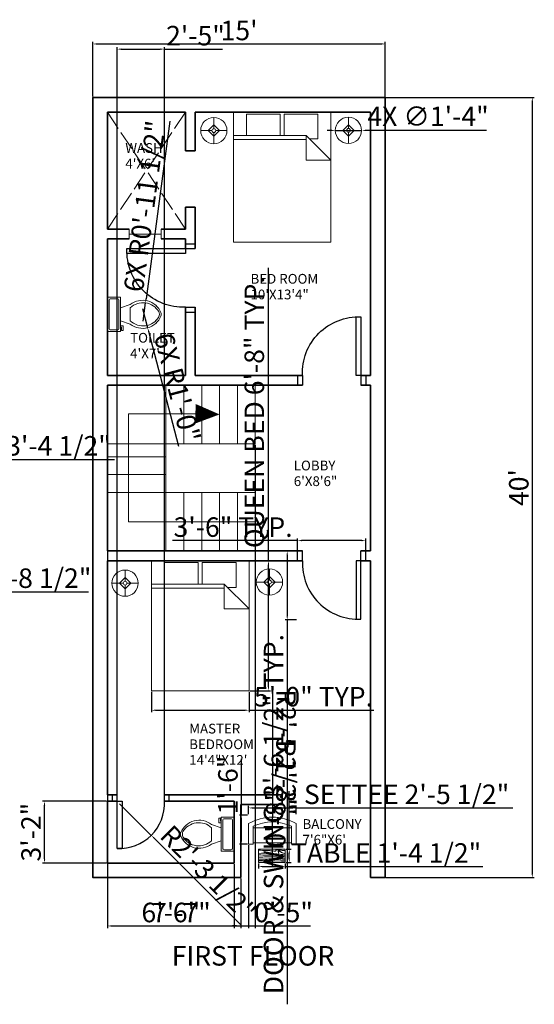
# Model space of a CAD drawing. Units: inches. Extents: x 2353 to 2961, y 642 to 1248.
# Tile 5 of 5: x 2644 to 2961, y 642 to 1248. Entities that reach past the tile are written whole.
import ezdxf

# ---------------------------------------------------------------- set-up
doc = ezdxf.new("R2010")
doc.units = ezdxf.units.IN
doc.linetypes.add('ACAD_ISO02W100', pattern=[15, 12, -3])
for name, color, linetype, lineweight in [('A-ANNO-DIMS', 2, 'Continuous', 18), ('A-ANNO-TEXT', 7, 'Continuous', 25), ('A-AREA-IDEN', 7, 'Continuous', 18), ('A-DOOR', 4, 'Continuous', 25), ('A-FLOR-FIXT', 9, 'Continuous', 18), ('A-FLOR-OPEN', 8, 'ACAD_ISO02W100', 13), ('A-FLOR-STRS', 7, 'Continuous', 18), ('A-FURN', 8, 'Continuous', 18), ('A-GLAZ', 4, 'Continuous', 18), ('A-WALL', 7, 'Continuous', 35)]:
    doc.layers.add(name, color=color, linetype=linetype, lineweight=lineweight)
doc.styles.get("Standard").update_dxf_attribs({"font": 'arial.ttf'})
doc.dimstyles.new('ISO-25', dxfattribs={"dimtxt": 12, "dimasz": 2.5, "dimexe": 1.25, "dimexo": 0.625, "dimtad": 1, "dimdec": 1, "dimlunit": 3, "dimtxsty": 'Standard', "dimcen": 2.5, "dimadec": 0, "dimazin": 0, "dimtfac": 1, "dimtdec": 1, "dimtmove": 0, "dimatfit": 3, "dimfxl": 1, "dimarcsym": 0})

# ---------------------------------------------------------------- blocks, each defined once
blk = doc.blocks.new('*D9')
at = {"layer": 'A-ANNO-DIMS', "color": 0, "lineweight": -2, "transparency": 16777216}
for p, q in [((2870.09, 1199.98), (2961.19, 1199.98)), ((2959.94, 1197.48), (2959.94, 722.48)), ((2870.09, 719.98), (2961.19, 719.98))]:
    blk.add_line(p, q, dxfattribs=at)
at = {"layer": 'A-ANNO-DIMS', "color": 0, "transparency": 16777216}
for points in [[(2959.53, 1197.48), (2960.36, 1197.48), (2959.94, 1199.98)], [(2959.53, 722.48), (2960.36, 722.48), (2959.94, 719.98)]]:
    blk.add_solid(points, dxfattribs=at)
at = {"layer": 'Defpoints', "color": 0, "transparency": 16777216}
for p in [(2869.46, 1199.98), (2869.46, 719.98), (2959.94, 719.98)]:
    blk.add_point(p, dxfattribs=at)
at = {"layer": 'A-ANNO-DIMS', "color": 0, "transparency": 16777216, "insert": (2953.19, 959.98), "char_height": 12, "attachment_point": 5, "rotation": 90}
blk.add_mtext("40'", dxfattribs=at)
blk = doc.blocks.new('Sofa - Roundback Loveseat 5 ft.')
for p, q in [((-24, -33.99998), (-24, -11.46958)), ((0, -32.44198), (0, -5.99998)), ((24.00004, -33.99998), (24.00004, -11.46958)), ((-23.9998, -13.38178), (23.99986, -13.38178)), ((-24, -32.44198), (24.00004, -32.44198))]:
    blk.add_line(p, q)
for points in [[(-24, -33.99998), (-30, -33.99998), (-30, -7.99998)], [(30.00004, -7.99998), (30.00004, -33.99998), (24.00004, -33.99998)]]:
    blk.add_lwpolyline(points)
for centre, radius, start, end in [((0, -60.24998), 60.24998, 60.13715, 119.8628), ((0, -61.38438), 55.38444, 64.32083, 115.6792)]:
    blk.add_arc(centre, radius, start, end)
blk = doc.blocks.new('Bed - Queen')
for p, q in [((0, -80.00003), (0, 0)), ((0, 0), (59.99999, 0)), ((59.99999, 0), (59.99999, -80.00003)), ((7.99999, -1.2), (28.79998, -1.2)), ((7.99999, -14.4), (7.99999, -1.2)), ((28.79998, -1.2), (28.79998, -14.4)), ((31.19999, -1.2), (51.99999, -1.2)), ((31.19999, -14.4), (31.19999, -1.2)), ((51.99999, -1.2), (51.99999, -16.4)), ((0, -14.4), (44.8, -14.4)), ((44.8, -16.8), (0, -16.8)), ((59.99999, -29.6), (44.8, -14.4)), ((44.8, -14.4), (44.8, -29.6)), ((51.99999, -16.4), (46.79936, -16.4)), ((44.8, -29.6), (59.99999, -29.6)), ((59.99999, -80.00003), (0, -80.00003))]:
    blk.add_line(p, q)
blk = doc.blocks.new('Lamp - Table')
for p, q in [((0, 7), (0, 1)), ((-1, 0), (-7, 0)), ((0, 3), (-3, 0)), ((-3, 0), (0, -3)), ((3, 0), (0, 3)), ((0, -3), (3, 0)), ((1, 0), (7, 0)), ((0, -1), (0, -7))]:
    blk.add_line(p, q)
for radius in [7, 1]:
    blk.add_circle((0, 0), radius)
blk = doc.blocks.new('Toilet - top')
for p, q in [((9.5, -6), (9.5, -2)), ((-10, -8.5), (-8, -8.5)), ((-10, -9.5), (-10, -8.5)), ((-7, -9.5), (-10, -9.5)), ((-8, -8.5), (-8, -8)), ((-7, -8), (-7, -9.5)), ((-4, -8), (-6, -14)), ((4, -8), (6, -14)), ((4, -14), (-4, -14))]:
    blk.add_line(p, q)
blk.add_lwpolyline([(10.5, -8), (10.5, 0), (-10.5, 0), (-10.5, -8)], close=True)
for points in [[(-9.5, -2), (-9.5, -6)], [(8.5, -1), (-8.5, -1)], [(-8.5, -7), (8.5, -7)]]:
    blk.add_lwpolyline(points)
for centre, radius, start, end in [((-8.62, -1.88), 0.884, 81.8699, 188.1301), ((-8.62, -6.12), 0.884, 171.8699, 278.1301), ((8.62, -1.88), 0.884, 351.8699, 98.1301), ((8.62, -6.12), 0.884, 261.8699, 8.1301), ((3.52, -21.58), 12.17, 141.46911, 247.97143), ((4.2, -21.82), 11.33, 136.36773, 238.94682), ((-3.52, -21.58), 12.17, 292.02843, 38.53071), ((-4.2, -21.82), 11.33, 301.05301, 43.63209), ((0, -27.88), 4, 245.73182, 294.26817), ((0, -29), 4, 254.86053, 285.13947)]:
    blk.add_arc(centre, radius, start, end)
blk = doc.blocks.new('Table - Rectangular Woodgrain 60 x 30 in.')
for p, q in [((0, 0), (0, -30)), ((60, 0), (0, 0)), ((60, -30), (60, 0)), ((0, -30), (60, -30))]:
    blk.add_line(p, q)
for points in [[(0, -2.4), (4.8155, -2.418), (9.0302, -2.4688), (12.709, -2.5477), (15.9167, -2.65), (18.7181, -2.7711), (21.1781, -2.9063), (23.3616, -3.0508), (25.3333, -3.2), (27.1477, -3.3495), (28.8172, -3.4958), (30.3437, -3.636), (31.7291, -3.7667), (32.9756, -3.8849), (34.0849, -3.9875), (35.059, -4.0714), (35.9, -4.1334), (36.6114, -4.1711), (37.2041, -4.1854), (37.6906, -4.1779), (38.0833, -4.15), (38.3948, -4.1034), (38.6375, -4.0396), (38.8239, -3.9602), (38.9666, -3.8667), (39.0764, -3.7608), (39.1573, -3.6448), (39.2116, -3.521), (39.2416, -3.3917), (39.2498, -3.2593), (39.2385, -3.1261), (39.21, -2.9944), (39.1666, -2.8667), (39.111, -2.7447), (39.0468, -2.6281), (38.978, -2.5163), (38.9083, -2.4083), (38.8418, -2.3035), (38.7823, -2.201), (38.7337, -2.1001), (38.7, -2), (38.6844, -1.9003), (38.6875, -1.8021), (38.7094, -1.707), (38.75, -1.6167), (38.8094, -1.5326), (38.8875, -1.4563), (38.9844, -1.3893), (39.1, -1.3333), (39.2351, -1.2896), (39.3937, -1.2583), (39.5804, -1.2396), (39.8, -1.2333), (40.057, -1.2396), (40.3562, -1.2583), (40.7023, -1.2896), (41.1, -1.3333), (41.5547, -1.3895), (42.0755, -1.4573), (42.6721, -1.5361), (43.3542, -1.625), (44.1316, -1.7233), (45.014, -1.8302), (46.0114, -1.9449), (47.1333, -2.0667), (48.3862, -2.1947), (49.7625, -2.3281), (51.2513, -2.4663), (52.8416, -2.6083), (54.5226, -2.7535), (56.2833, -2.9011), (58.1127, -3.0501), (60, -3.2)], [(0, -9.2), (6.5759, -9.0858), (11.9385, -9.0365), (16.2527, -9.0418), (19.6833, -9.0917), (22.3952, -9.1759), (24.5531, -9.2844), (26.322, -9.4069), (27.8666, -9.5333), (29.3241, -9.6553), (30.7203, -9.7719), (32.0532, -9.8837), (33.3208, -9.9917), (34.5213, -10.0965), (35.6526, -10.199), (36.7128, -10.2999), (37.7, -10.4), (38.6129, -10.4996), (39.4531, -10.5969), (40.223, -10.6895), (40.925, -10.775), (41.5613, -10.8512), (42.1344, -10.9156), (42.6465, -10.966), (43.1, -11), (43.4976, -11.0158), (43.8437, -11.0136), (44.143, -10.9942), (44.4, -10.9583), (44.6195, -10.9069), (44.8062, -10.8406), (44.9648, -10.7603), (45.1, -10.6667), (45.2155, -10.5598), (45.3114, -10.4365), (45.3871, -10.2929), (45.4416, -10.125), (45.4743, -9.929), (45.4844, -9.7011), (45.4709, -9.4371), (45.4333, -9.1333), (45.3716, -8.7883), (45.2896, -8.4104), (45.1919, -8.0107), (45.0833, -7.6), (44.9685, -7.1893), (44.8521, -6.7896), (44.7388, -6.4117), (44.6333, -6.0667), (44.54, -5.7628), (44.4614, -5.4979), (44.4001, -5.2675), (44.3583, -5.0667), (44.3384, -4.8909), (44.3427, -4.7354), (44.3736, -4.5956), (44.4333, -4.4667), (44.5236, -4.3453), (44.6427, -4.2333), (44.7884, -4.1339), (44.9583, -4.05), (45.1501, -3.9849), (45.3614, -3.9417), (45.59, -3.9234), (45.8333, -3.9333), (46.0915, -3.9749), (46.3734, -4.0531), (46.6906, -4.1736), (47.0542, -4.3417), (47.4756, -4.5629), (47.9661, -4.8427), (48.5372, -5.1866), (49.2, -5.6), (49.9676, -6.0844), (50.8594, -6.625), (51.8965, -7.2031), (53.1, -7.8), (54.491, -8.3969), (56.0906, -8.975), (57.9199, -9.5156), (60, -10)], [(0, -12.8), (5.1847, -12.9322), (9.6213, -13.0323), (13.3963, -13.1059), (16.5958, -13.1583), (19.3063, -13.1952), (21.614, -13.2219), (23.6054, -13.2439), (25.3666, -13.2667), (26.9728, -13.2947), (28.4531, -13.3281), (29.8256, -13.3663), (31.1083, -13.4083), (32.3191, -13.4535), (33.476, -13.501), (34.597, -13.5501), (35.7, -13.6), (36.7984, -13.6497), (37.8875, -13.6979), (38.9578, -13.743), (40, -13.7833), (41.0047, -13.8174), (41.9625, -13.8438), (42.864, -13.8607), (43.7, -13.8667), (44.4631, -13.8604), (45.1552, -13.8417), (45.7801, -13.8104), (46.3416, -13.7667), (46.8439, -13.7104), (47.2906, -13.6417), (47.6858, -13.5604), (48.0333, -13.4667), (48.3375, -13.3608), (48.6042, -13.2448), (48.8396, -13.121), (49.05, -12.9917), (49.2417, -12.8593), (49.4208, -12.7261), (49.5937, -12.5944), (49.7667, -12.4667), (49.9452, -12.3451), (50.1323, -12.2313), (50.3303, -12.1268), (50.5416, -12.0333), (50.7686, -11.9524), (51.0135, -11.8854), (51.2788, -11.8341), (51.5666, -11.8), (51.8785, -11.7843), (52.2116, -11.7865), (52.562, -11.8059), (52.926, -11.8417), (53.2998, -11.8931), (53.6795, -11.9594), (54.0614, -12.0397), (54.4416, -12.1333), (54.8223, -12.2401), (55.2293, -12.3625), (55.6942, -12.5037), (56.2489, -12.6667), (56.9251, -12.8547), (57.7545, -13.0708), (58.7689, -13.3182), (60, -13.6)], [(0, -18), (5.124, -17.7273), (9.6609, -17.5057), (13.6705, -17.3303), (17.2125, -17.1958), (20.3467, -17.0973), (23.1328, -17.0297), (25.6307, -16.9878), (27.9, -16.9667), (29.9928, -16.9617), (31.9302, -16.9703), (33.7254, -16.9907), (35.3917, -17.0208), (36.9423, -17.0588), (38.3906, -17.1026), (39.7499, -17.1503), (41.0333, -17.2), (42.2519, -17.2496), (43.4073, -17.2969), (44.4986, -17.3395), (45.525, -17.375), (46.4858, -17.4012), (47.3802, -17.4156), (48.2074, -17.416), (48.9667, -17.4), (49.6583, -17.3662), (50.2872, -17.3167), (50.8595, -17.2547), (51.3812, -17.1833), (51.8584, -17.1057), (52.2971, -17.025), (52.7034, -16.9443), (53.0833, -16.8667), (53.443, -16.7951), (53.789, -16.7313), (54.128, -16.6768), (54.4666, -16.6334), (54.8115, -16.6024), (55.1693, -16.5854), (55.5465, -16.5841), (55.95, -16.6), (56.3828, -16.6337), (56.8346, -16.6823), (57.2915, -16.7418), (57.7396, -16.8084), (58.165, -16.878), (58.5539, -16.9469), (58.8924, -17.0111), (59.1666, -17.0667), (59.3679, -17.1107), (59.5078, -17.1438), (59.6032, -17.1675), (59.6708, -17.1833), (59.7275, -17.193), (59.7901, -17.1979), (59.8753, -17.1998), (60, -17.2)], [(0, -22.4), (8.0098, -22.2501), (14.4094, -22.1011), (19.4168, -21.9535), (23.25, -21.8083), (26.1269, -21.6663), (28.2656, -21.5281), (29.884, -21.3947), (31.2, -21.2667), (32.3967, -21.1448), (33.5172, -21.0292), (34.5697, -20.9198), (35.5625, -20.8167), (36.5037, -20.7198), (37.4015, -20.6292), (38.2642, -20.5448), (39.1, -20.4667), (39.9164, -20.3951), (40.7187, -20.3313), (41.5117, -20.2768), (42.3, -20.2333), (43.0883, -20.2024), (43.8812, -20.1854), (44.6836, -20.1841), (45.5, -20.2), (46.3328, -20.234), (47.1747, -20.2844), (48.0163, -20.3488), (48.8479, -20.425), (49.66, -20.5106), (50.4429, -20.6031), (51.1872, -20.7004), (51.8833, -20.8), (52.5246, -20.8999), (53.1166, -20.9995), (53.6681, -21.0983), (54.1875, -21.1958), (54.6834, -21.2919), (55.1646, -21.3859), (55.6394, -21.4777), (56.1167, -21.5667), (56.6028, -21.6515), (57.0961, -21.7266), (57.5929, -21.7852), (58.0896, -21.8208), (58.5823, -21.8268), (59.0674, -21.7964), (59.5412, -21.723), (60, -21.6)], [(0, -25.2), (8.6355, -25.0504), (15.7026, -24.9031), (21.4049, -24.7606), (25.9458, -24.625), (29.529, -24.4988), (32.3578, -24.3844), (34.6359, -24.284), (36.5667, -24.2), (38.3213, -24.1341), (39.9417, -24.0854), (41.437, -24.0523), (42.8167, -24.0333), (44.0901, -24.0268), (45.2667, -24.0313), (46.3557, -24.0451), (47.3667, -24.0667), (48.309, -24.0947), (49.1928, -24.1287), (50.0284, -24.168), (50.826, -24.2125), (51.5959, -24.2617), (52.3483, -24.3151), (53.0935, -24.3725), (53.8417, -24.4334), (54.6009, -24.497), (55.3699, -24.561), (56.1454, -24.6226), (56.9239, -24.6792), (57.7021, -24.7279), (58.4764, -24.7662), (59.2435, -24.7911), (60, -24.8)], [(0, -28.8), (5.6867, -28.6681), (10.45, -28.5698), (14.407, -28.5012), (17.675, -28.4584), (20.3711, -28.4374), (22.6125, -28.4344), (24.5164, -28.4455), (26.2, -28.4667), (27.762, -28.4947), (29.2276, -28.5281), (30.6033, -28.5663), (31.8958, -28.6084), (33.1118, -28.6535), (34.2578, -28.7011), (35.3405, -28.7501), (36.3666, -28.8), (37.3443, -28.8497), (38.288, -28.8974), (39.2137, -28.9412), (40.1375, -28.9792), (41.0753, -29.0093), (42.0432, -29.0297), (43.0572, -29.0384), (44.1333, -29.0333), (45.2936, -29.0114), (46.5843, -28.9641), (48.0579, -28.8816), (49.7666, -28.7542), (51.7629, -28.5721), (54.0989, -28.3255), (56.8272, -28.0048), (60, -27.6)]]:
    blk.add_lwpolyline(points)
blk = doc.blocks.new('*D11')
at = {"layer": 'A-ANNO-DIMS', "color": 0, "lineweight": -2, "transparency": 16777216}
for p, q in [((2689.46, 1200.61), (2689.46, 1234.16)), ((2691.96, 1232.91), (2866.96, 1232.91)), ((2869.46, 1200.61), (2869.46, 1234.16))]:
    blk.add_line(p, q, dxfattribs=at)
at = {"layer": 'A-ANNO-DIMS', "color": 0, "transparency": 16777216}
for points in [[(2691.96, 1233.33), (2691.96, 1232.49), (2689.46, 1232.91)], [(2866.96, 1233.33), (2866.96, 1232.49), (2869.46, 1232.91)]]:
    blk.add_solid(points, dxfattribs=at)
at = {"layer": 'Defpoints', "color": 0, "transparency": 16777216}
for p in [(2869.46, 1232.91), (2689.46, 1199.98), (2869.46, 1199.98)]:
    blk.add_point(p, dxfattribs=at)
at = {"layer": 'A-ANNO-DIMS', "color": 0, "transparency": 16777216, "insert": (2779.46, 1239.66), "char_height": 12, "attachment_point": 5}
blk.add_mtext("15'", dxfattribs=at)
blk = doc.blocks.new('DOOR-SINGLE-36IN')
for p, q in [((0, 6), (0, 0)), ((3, 6), (3, 0)), ((39, 6), (39, 0)), ((42, 6), (42, 0))]:
    blk.add_line(p, q)
blk.add_lwpolyline([(3, 6), (6, 6), (6, 42), (3, 42)], close=True)
blk.add_arc((4.5, 7.5), 34.53, 357.51045, 92.48955)
blk = doc.blocks.new('WASH-COURT-CROSS-4X6')
for p, q in [((0, 72), (48, 0)), ((48, 72), (0, 0))]:
    blk.add_line(p, q)
blk = doc.blocks.new('*D15')
at = {"layer": 'A-ANNO-DIMS', "color": 0, "lineweight": -2, "transparency": 16777216}
for p, q in [((2814.84, 920.98), (2807.85, 920.98)), ((2809.1, 918.48), (2809.1, 881.06)), ((2814.84, 878.56), (2807.85, 878.56)), ((2809.1, 878.56), (2809.1, 642.05))]:
    blk.add_line(p, q, dxfattribs=at)
at = {"layer": 'A-ANNO-DIMS', "color": 0, "transparency": 16777216}
for points in [[(2808.69, 918.48), (2809.52, 918.48), (2809.1, 920.98)], [(2808.69, 881.06), (2809.52, 881.06), (2809.1, 878.56)]]:
    blk.add_solid(points, dxfattribs=at)
at = {"layer": 'Defpoints', "color": 0, "transparency": 16777216}
for p in [(2815.46, 920.98), (2809.1, 878.56), (2815.46, 878.56)]:
    blk.add_point(p, dxfattribs=at)
at = {"layer": 'A-ANNO-DIMS', "color": 0, "transparency": 16777216, "insert": (2802.23, 759.06), "char_height": 12, "attachment_point": 5, "rotation": 90}
blk.add_mtext('DOOR & SWING 3\'-6 1/2" TYP.', dxfattribs=at)
blk = doc.blocks.new('*D16')
at = {"layer": 'A-ANNO-DIMS', "color": 0, "lineweight": -2, "transparency": 16777216}
for p, q in [((2815.46, 927.35), (2738.58, 927.35)), ((2815.46, 921.61), (2815.46, 928.6)), ((2854.96, 927.35), (2817.96, 927.35)), ((2857.46, 921.61), (2857.46, 928.6))]:
    blk.add_line(p, q, dxfattribs=at)
at = {"layer": 'A-ANNO-DIMS', "color": 0, "transparency": 16777216}
for points in [[(2817.96, 927.76), (2817.96, 926.93), (2815.46, 927.35)], [(2854.96, 927.76), (2854.96, 926.93), (2857.46, 927.35)]]:
    blk.add_solid(points, dxfattribs=at)
at = {"layer": 'Defpoints', "color": 0, "transparency": 16777216}
for p in [(2815.46, 927.35), (2815.46, 920.98), (2857.46, 920.98)]:
    blk.add_point(p, dxfattribs=at)
at = {"layer": 'A-ANNO-DIMS', "color": 0, "transparency": 16777216, "insert": (2775.77, 934.1), "char_height": 12, "attachment_point": 5}
blk.add_mtext('3\'-6" TYP.', dxfattribs=at)
blk = doc.blocks.new('*D17')
at = {"layer": 'A-ANNO-DIMS', "color": 0, "lineweight": -2, "transparency": 16777216}
for p, q in [((2797.58, 914.98), (2797.58, 1095.26)), ((2786.2, 914.98), (2798.83, 914.98)), ((2797.58, 837.48), (2797.58, 912.48)), ((2786.2, 834.98), (2798.83, 834.98))]:
    blk.add_line(p, q, dxfattribs=at)
at = {"layer": 'A-ANNO-DIMS', "color": 0, "transparency": 16777216}
for points in [[(2797.16, 912.48), (2797.99, 912.48), (2797.58, 914.98)], [(2797.16, 837.48), (2797.99, 837.48), (2797.58, 834.98)]]:
    blk.add_solid(points, dxfattribs=at)
at = {"layer": 'Defpoints', "color": 0, "transparency": 16777216}
for p in [(2785.58, 914.98), (2797.58, 914.98), (2785.58, 834.98)]:
    blk.add_point(p, dxfattribs=at)
at = {"layer": 'A-ANNO-DIMS', "color": 0, "transparency": 16777216, "insert": (2790.38, 1006.37), "char_height": 12, "attachment_point": 5, "rotation": 90}
blk.add_mtext('QUEEN BED 6\'-8" TYP.', dxfattribs=at)
blk = doc.blocks.new('*D18')
at = {"layer": 'A-ANNO-DIMS', "color": 0, "lineweight": -2, "transparency": 16777216}
for p, q in [((2725.58, 834.36), (2725.58, 821.73)), ((2785.58, 834.36), (2785.58, 821.73)), ((2728.08, 822.98), (2783.08, 822.98)), ((2785.58, 822.98), (2862.47, 822.98))]:
    blk.add_line(p, q, dxfattribs=at)
at = {"layer": 'A-ANNO-DIMS', "color": 0, "transparency": 16777216}
for points in [[(2728.08, 823.4), (2728.08, 822.57), (2725.58, 822.98)], [(2783.08, 823.4), (2783.08, 822.57), (2785.58, 822.98)]]:
    blk.add_solid(points, dxfattribs=at)
at = {"layer": 'Defpoints', "color": 0, "transparency": 16777216}
for p in [(2725.58, 834.98), (2785.58, 834.98), (2785.58, 822.98)]:
    blk.add_point(p, dxfattribs=at)
at = {"layer": 'A-ANNO-DIMS', "color": 0, "transparency": 16777216, "insert": (2825.27, 829.74), "char_height": 12, "attachment_point": 5}
blk.add_mtext('5\'-0" TYP.', dxfattribs=at)
blk = doc.blocks.new('*D21')
at = {"layer": 'A-ANNO-DIMS', "color": 0, "lineweight": -2, "transparency": 16777216}
for p, q in [((2529.01, 971.84), (2529.01, 978.53)), ((2531.51, 977.28), (2566.89, 977.28)), ((2569.39, 971.84), (2569.39, 978.53)), ((2569.39, 977.28), (2702.81, 977.28))]:
    blk.add_line(p, q, dxfattribs=at)
at = {"layer": 'A-ANNO-DIMS', "color": 0, "transparency": 16777216}
for points in [[(2531.51, 977.69), (2531.51, 976.86), (2529.01, 977.28)], [(2566.89, 977.69), (2566.89, 976.86), (2569.39, 977.28)]]:
    blk.add_solid(points, dxfattribs=at)
at = {"layer": 'Defpoints', "color": 0, "transparency": 16777216}
for p in [(2569.39, 977.28), (2529.01, 971.22), (2569.39, 971.22)]:
    blk.add_point(p, dxfattribs=at)
at = {"layer": 'A-ANNO-DIMS', "color": 0, "transparency": 16777216, "insert": (2637.35, 984.11), "char_height": 12, "attachment_point": 5}
blk.add_mtext('SETTEE 3\'-4 1/2"', dxfattribs=at)
blk = doc.blocks.new('*D23')
at = {"layer": 'A-ANNO-DIMS', "color": 0, "lineweight": -2, "transparency": 16777216}
for p, q in [((2785.29, 759.09), (2785.29, 764.12)), ((2814.63, 759.09), (2814.63, 764.12)), ((2787.79, 762.87), (2812.13, 762.87)), ((2814.63, 762.87), (2948.05, 762.87))]:
    blk.add_line(p, q, dxfattribs=at)
at = {"layer": 'A-ANNO-DIMS', "color": 0, "transparency": 16777216}
for points in [[(2787.79, 763.28), (2787.79, 762.45), (2785.29, 762.87)], [(2812.13, 763.28), (2812.13, 762.45), (2814.63, 762.87)]]:
    blk.add_solid(points, dxfattribs=at)
at = {"layer": 'Defpoints', "color": 0, "transparency": 16777216}
for p in [(2785.29, 758.46), (2814.63, 762.87), (2814.63, 758.46)]:
    blk.add_point(p, dxfattribs=at)
at = {"layer": 'A-ANNO-DIMS', "color": 0, "transparency": 16777216, "insert": (2882.59, 769.7), "char_height": 12, "attachment_point": 5}
blk.add_mtext('SETTEE 2\'-5 1/2"', dxfattribs=at)
blk = doc.blocks.new('*D24')
at = {"layer": 'A-ANNO-DIMS', "color": 0, "lineweight": -2, "transparency": 16777216}
for p, q in [((2780.89, 758.46), (2780.89, 792.98)), ((2784.67, 758.46), (2779.64, 758.46)), ((2780.89, 743.03), (2780.89, 755.96)), ((2784.67, 740.53), (2779.64, 740.53))]:
    blk.add_line(p, q, dxfattribs=at)
at = {"layer": 'A-ANNO-DIMS', "color": 0, "transparency": 16777216}
for points in [[(2780.47, 755.96), (2781.31, 755.96), (2780.89, 758.46)], [(2780.47, 743.03), (2781.31, 743.03), (2780.89, 740.53)]]:
    blk.add_solid(points, dxfattribs=at)
at = {"layer": 'Defpoints', "color": 0, "transparency": 16777216}
for p in [(2780.89, 758.46), (2785.29, 758.46), (2785.29, 740.53)]:
    blk.add_point(p, dxfattribs=at)
at = {"layer": 'A-ANNO-DIMS', "color": 0, "transparency": 16777216, "insert": (2774.14, 776.97), "char_height": 12, "attachment_point": 5, "rotation": 90}
blk.add_mtext('1\'-6"', dxfattribs=at)
blk = doc.blocks.new('*D27')
at = {"layer": 'A-ANNO-DIMS', "color": 0, "lineweight": -2, "transparency": 16777216}
for p, q in [((2791.43, 728.61), (2791.43, 725.52)), ((2807.88, 728.61), (2807.88, 725.52)), ((2793.93, 726.77), (2805.38, 726.77)), ((2807.88, 726.77), (2929.56, 726.77))]:
    blk.add_line(p, q, dxfattribs=at)
at = {"layer": 'A-ANNO-DIMS', "color": 0, "transparency": 16777216}
for points in [[(2793.93, 727.19), (2793.93, 726.35), (2791.43, 726.77)], [(2805.38, 727.19), (2805.38, 726.35), (2807.88, 726.77)]]:
    blk.add_solid(points, dxfattribs=at)
at = {"layer": 'Defpoints', "color": 0, "transparency": 16777216}
for p in [(2791.43, 729.24), (2807.88, 729.24), (2807.88, 726.77)]:
    blk.add_point(p, dxfattribs=at)
at = {"layer": 'A-ANNO-DIMS', "color": 0, "transparency": 16777216, "insert": (2869.97, 733.6), "char_height": 12, "attachment_point": 5}
blk.add_mtext('TABLE 1\'-4 1/2"', dxfattribs=at)
blk = doc.blocks.new('*D28')
at = {"layer": 'A-ANNO-DIMS', "color": 0, "lineweight": -2, "transparency": 16777216}
for p, q in [((2810.35, 737.46), (2810.35, 773.11)), ((2808.5, 737.46), (2811.6, 737.46)), ((2810.35, 731.74), (2810.35, 734.96)), ((2808.5, 729.24), (2811.6, 729.24))]:
    blk.add_line(p, q, dxfattribs=at)
at = {"layer": 'A-ANNO-DIMS', "color": 0, "transparency": 16777216}
for points in [[(2809.93, 734.96), (2810.76, 734.96), (2810.35, 737.46)], [(2809.93, 731.74), (2810.76, 731.74), (2810.35, 729.24)]]:
    blk.add_solid(points, dxfattribs=at)
at = {"layer": 'Defpoints', "color": 0, "transparency": 16777216}
for p in [(2807.88, 737.46), (2810.35, 737.46), (2807.88, 729.24)]:
    blk.add_point(p, dxfattribs=at)
at = {"layer": 'A-ANNO-DIMS', "color": 0, "transparency": 16777216, "insert": (2803.6, 756.54), "char_height": 12, "attachment_point": 5, "rotation": 90}
blk.add_mtext('0\'-8"', dxfattribs=at)
blk = doc.blocks.new('*D33')
at = {"layer": 'A-ANNO-DIMS', "color": 0, "lineweight": -2, "transparency": 16777216}
for p, q in [((2698.46, 728.36), (2698.46, 688.98)), ((2776.46, 728.36), (2776.46, 688.98)), ((2700.96, 690.23), (2773.96, 690.23))]:
    blk.add_line(p, q, dxfattribs=at)
at = {"layer": 'A-ANNO-DIMS', "color": 0, "transparency": 16777216}
for points in [[(2700.96, 690.65), (2700.96, 689.82), (2698.46, 690.23)], [(2773.96, 690.65), (2773.96, 689.82), (2776.46, 690.23)]]:
    blk.add_solid(points, dxfattribs=at)
at = {"layer": 'Defpoints', "color": 0, "transparency": 16777216}
for p in [(2698.46, 728.98), (2776.46, 728.98), (2776.46, 690.23)]:
    blk.add_point(p, dxfattribs=at)
at = {"layer": 'A-ANNO-DIMS', "color": 0, "transparency": 16777216, "insert": (2737.46, 696.99), "char_height": 12, "attachment_point": 5}
blk.add_mtext('6\'-6"', dxfattribs=at)
blk = doc.blocks.new('*D34')
at = {"layer": 'A-ANNO-DIMS', "color": 0, "lineweight": -2, "transparency": 16777216}
for p, q in [((2697.84, 766.98), (2658.46, 766.98)), ((2659.71, 731.48), (2659.71, 764.48)), ((2697.84, 728.98), (2658.46, 728.98))]:
    blk.add_line(p, q, dxfattribs=at)
at = {"layer": 'A-ANNO-DIMS', "color": 0, "transparency": 16777216}
for points in [[(2659.3, 764.48), (2660.13, 764.48), (2659.71, 766.98)], [(2659.3, 731.48), (2660.13, 731.48), (2659.71, 728.98)]]:
    blk.add_solid(points, dxfattribs=at)
at = {"layer": 'Defpoints', "color": 0, "transparency": 16777216}
for p in [(2659.71, 766.98), (2698.46, 766.98), (2698.46, 728.98)]:
    blk.add_point(p, dxfattribs=at)
at = {"layer": 'A-ANNO-DIMS', "color": 0, "transparency": 16777216, "insert": (2652.96, 747.98), "char_height": 12, "attachment_point": 5, "rotation": 90}
blk.add_mtext('3\'-2"', dxfattribs=at)
blk = doc.blocks.new('*D37')
at = {"layer": 'A-ANNO-DIMS', "color": 0, "lineweight": -2, "transparency": 16777216}
for p, q in [((2698.46, 986.36), (2698.46, 688.98)), ((2789.46, 986.36), (2789.46, 688.98)), ((2700.96, 690.23), (2786.96, 690.23))]:
    blk.add_line(p, q, dxfattribs=at)
at = {"layer": 'A-ANNO-DIMS', "color": 0, "transparency": 16777216}
for points in [[(2700.96, 690.65), (2700.96, 689.82), (2698.46, 690.23)], [(2786.96, 690.65), (2786.96, 689.82), (2789.46, 690.23)]]:
    blk.add_solid(points, dxfattribs=at)
at = {"layer": 'Defpoints', "color": 0, "transparency": 16777216}
for p in [(2698.46, 986.98), (2789.46, 986.98), (2789.46, 690.23)]:
    blk.add_point(p, dxfattribs=at)
at = {"layer": 'A-ANNO-DIMS', "color": 0, "transparency": 16777216, "insert": (2743.96, 696.86), "char_height": 12, "attachment_point": 5}
blk.add_mtext('7\'-7"', dxfattribs=at)
blk = doc.blocks.new('*D39')
at = {"layer": 'A-ANNO-DIMS', "color": 0, "lineweight": -2, "transparency": 16777216}
for p, q in [((2704.46, 767.61), (2704.46, 1230.98)), ((2733.46, 767.61), (2733.46, 1230.98)), ((2706.96, 1229.73), (2730.96, 1229.73)), ((2733.46, 1229.73), (2769.32, 1229.73))]:
    blk.add_line(p, q, dxfattribs=at)
at = {"layer": 'A-ANNO-DIMS', "color": 0, "transparency": 16777216}
for points in [[(2706.96, 1230.15), (2706.96, 1229.32), (2704.46, 1229.73)], [(2730.96, 1230.15), (2730.96, 1229.32), (2733.46, 1229.73)]]:
    blk.add_solid(points, dxfattribs=at)
at = {"layer": 'Defpoints', "color": 0, "transparency": 16777216}
for p in [(2733.46, 1229.73), (2704.46, 766.98), (2733.46, 766.98)]:
    blk.add_point(p, dxfattribs=at)
at = {"layer": 'A-ANNO-DIMS', "color": 0, "transparency": 16777216, "insert": (2752.64, 1236.49), "char_height": 12, "attachment_point": 5}
blk.add_mtext('2\'-5"', dxfattribs=at)
blk = doc.blocks.new('*D41')
at = {"layer": 'A-ANNO-DIMS', "color": 0, "lineweight": -2, "transparency": 16777216}
for p, q in [((2785.29, 739.91), (2785.29, 688.98)), ((2780.46, 719.36), (2780.46, 688.98)), ((2777.96, 690.23), (2775.46, 690.23)), ((2780.46, 690.23), (2785.29, 690.23)), ((2787.79, 690.23), (2823.44, 690.23))]:
    blk.add_line(p, q, dxfattribs=at)
at = {"layer": 'A-ANNO-DIMS', "color": 0, "transparency": 16777216}
for points in [[(2777.96, 690.65), (2777.96, 689.82), (2780.46, 690.23)], [(2787.79, 690.65), (2787.79, 689.82), (2785.29, 690.23)]]:
    blk.add_solid(points, dxfattribs=at)
at = {"layer": 'Defpoints', "color": 0, "transparency": 16777216}
for p in [(2785.29, 740.53), (2780.46, 719.98), (2785.29, 690.23)]:
    blk.add_point(p, dxfattribs=at)
at = {"layer": 'A-ANNO-DIMS', "color": 0, "transparency": 16777216, "insert": (2806.87, 696.99), "char_height": 12, "attachment_point": 5}
blk.add_mtext('0\'-5"', dxfattribs=at)
blk = doc.blocks.new('*D42')
at = {"layer": 'A-ANNO-DIMS', "color": 0, "lineweight": -2, "transparency": 16777216}
for p, q in [((2571.41, 895.53), (2568.91, 895.53)), ((2573.91, 895.53), (2582.35, 895.54)), ((2686.86, 895.61), (2584.85, 895.54))]:
    blk.add_line(p, q, dxfattribs=at)
at = {"layer": 'A-ANNO-DIMS', "color": 0, "transparency": 16777216}
for points in [[(2571.41, 895.95), (2571.41, 895.12), (2573.91, 895.53)], [(2584.85, 895.96), (2584.85, 895.13), (2582.35, 895.54)]]:
    blk.add_solid(points, dxfattribs=at)
at = {"layer": 'Defpoints', "color": 0, "transparency": 16777216}
for p in [(2573.91, 895.53), (2582.35, 895.54)]:
    blk.add_point(p, dxfattribs=at)
at = {"layer": 'A-ANNO-DIMS', "color": 0, "transparency": 16777216, "insert": (2637.1, 902.66), "char_height": 12, "attachment_point": 5, "rotation": 0.03863}
blk.add_mtext('2X ∅0\'-8 1/2"', dxfattribs=at)
blk = doc.blocks.new('*D43')
at = {"layer": 'A-ANNO-DIMS', "color": 0, "lineweight": -2, "transparency": 16777216}
for p, q in [((2836.19, 1179.73), (2833.69, 1179.73)), ((2838.69, 1179.73), (2854.86, 1179.73)), ((2931.7, 1179.73), (2857.36, 1179.73))]:
    blk.add_line(p, q, dxfattribs=at)
at = {"layer": 'A-ANNO-DIMS', "color": 0, "transparency": 16777216}
for points in [[(2836.19, 1180.15), (2836.19, 1179.32), (2838.69, 1179.73)], [(2857.36, 1180.15), (2857.36, 1179.32), (2854.86, 1179.73)]]:
    blk.add_solid(points, dxfattribs=at)
at = {"layer": 'Defpoints', "color": 0, "transparency": 16777216}
for p in [(2838.69, 1179.73), (2854.86, 1179.73)]:
    blk.add_point(p, dxfattribs=at)
at = {"layer": 'A-ANNO-DIMS', "color": 0, "transparency": 16777216, "insert": (2895.78, 1186.82), "char_height": 12, "attachment_point": 5, "rotation": 359.99946}
blk.add_mtext('4X ∅1\'-4"', dxfattribs=at)
blk = doc.blocks.new('*D45')
at = {"layer": 'A-ANNO-DIMS', "color": 0, "lineweight": -2, "transparency": 16777216}
for p, q in [((2705.96, 765.48), (2725.44, 746.01)), ((2780.31, 691.14), (2727.21, 744.24))]:
    blk.add_line(p, q, dxfattribs=at)
at = {"layer": 'A-ANNO-DIMS', "color": 0, "transparency": 16777216}
blk.add_solid([(2727.5, 744.54), (2726.91, 743.95), (2725.44, 746.01)], dxfattribs=at)
at = {"layer": 'Defpoints', "color": 0, "transparency": 16777216}
for p in [(2705.96, 765.48), (2725.44, 746.01)]:
    blk.add_point(p, dxfattribs=at)
at = {"layer": 'A-ANNO-DIMS', "color": 0, "transparency": 16777216, "insert": (2759.47, 721.64), "char_height": 12, "attachment_point": 5, "rotation": 315.00016}
blk.add_mtext('R2\'-3 1/2"', dxfattribs=at)
blk = doc.blocks.new('*D50')
at = {"layer": 'A-ANNO-DIMS', "color": 0, "lineweight": -2, "transparency": 16777216}
for p, q in [((2799.96, 834.76), (2799.96, 759.66)), ((2799.96, 727.7), (2799.96, 757.16))]:
    blk.add_line(p, q, dxfattribs=at)
at = {"layer": 'A-ANNO-DIMS', "color": 0, "transparency": 16777216}
blk.add_solid([(2800.38, 759.66), (2799.55, 759.66), (2799.96, 757.16)], dxfattribs=at)
at = {"layer": 'Defpoints', "color": 0, "transparency": 16777216}
for p in [(2799.96, 757.16), (2799.96, 727.7)]:
    blk.add_point(p, dxfattribs=at)
at = {"layer": 'A-ANNO-DIMS', "color": 0, "transparency": 16777216, "insert": (2806.79, 798.46), "char_height": 12, "attachment_point": 5, "rotation": 270.00075}
blk.add_mtext('R2\'-5 1/2"', dxfattribs=at)
blk = doc.blocks.new('*D51')
at = {"layer": 'A-ANNO-DIMS', "color": 0, "lineweight": -2, "transparency": 16777216}
for p, q in [((2799.96, 803.86), (2799.96, 756.73)), ((2799.96, 727.14), (2799.96, 754.23))]:
    blk.add_line(p, q, dxfattribs=at)
at = {"layer": 'A-ANNO-DIMS', "color": 0, "transparency": 16777216}
blk.add_solid([(2800.38, 756.73), (2799.55, 756.73), (2799.96, 754.23)], dxfattribs=at)
at = {"layer": 'Defpoints', "color": 0, "transparency": 16777216}
for p in [(2799.96, 754.23), (2799.96, 727.14)]:
    blk.add_point(p, dxfattribs=at)
at = {"layer": 'A-ANNO-DIMS', "color": 0, "transparency": 16777216, "insert": (2806.72, 781.54), "char_height": 12, "attachment_point": 5, "rotation": 270.00082}
blk.add_mtext('R2\'-3"', dxfattribs=at)
blk = doc.blocks.new('*D52')
at = {"layer": 'A-ANNO-DIMS', "color": 0, "lineweight": -2, "transparency": 16777216}
for p, q in [((2720.1, 1070.09), (2723.19, 1058.32)), ((2742.37, 985.31), (2723.83, 1055.9))]:
    blk.add_line(p, q, dxfattribs=at)
at = {"layer": 'A-ANNO-DIMS', "color": 0, "transparency": 16777216}
blk.add_solid([(2724.23, 1056.01), (2723.42, 1055.8), (2723.19, 1058.32)], dxfattribs=at)
at = {"layer": 'Defpoints', "color": 0, "transparency": 16777216}
for p in [(2720.1, 1070.09), (2723.19, 1058.32)]:
    blk.add_point(p, dxfattribs=at)
at = {"layer": 'A-ANNO-DIMS', "color": 0, "transparency": 16777216, "insert": (2739.95, 1021.12), "char_height": 12, "attachment_point": 5, "rotation": 284.72023}
blk.add_mtext('6X R1\'-0"', dxfattribs=at)
blk = doc.blocks.new('*D53')
at = {"layer": 'A-ANNO-DIMS', "color": 0, "lineweight": -2, "transparency": 16777216}
for p, q in [((2736.87, 1185.36), (2722.18, 1076.08)), ((2720.33, 1062.37), (2721.84, 1073.6))]:
    blk.add_line(p, q, dxfattribs=at)
at = {"layer": 'A-ANNO-DIMS', "color": 0, "transparency": 16777216}
blk.add_solid([(2721.76, 1076.13), (2722.59, 1076.02), (2721.84, 1073.6)], dxfattribs=at)
at = {"layer": 'Defpoints', "color": 0, "transparency": 16777216}
for p in [(2721.84, 1073.6), (2720.33, 1062.37)]:
    blk.add_point(p, dxfattribs=at)
at = {"layer": 'A-ANNO-DIMS', "color": 0, "transparency": 16777216, "insert": (2722.92, 1132.87), "char_height": 12, "attachment_point": 5, "rotation": 82.3437}
blk.add_mtext('6X R0\'-11 1/2"', dxfattribs=at)

msp = doc.modelspace()

# ---------------------------------------------------------------- linework, layer by layer
at = {"layer": 'A-DOOR'}
for p, q in [((2701.46, 766.98), (2701.46, 770.98)), ((2704.46, 766.98), (2704.46, 770.98)), ((2733.46, 766.98), (2733.46, 770.98)), ((2736.46, 766.98), (2736.46, 770.98))]:
    msp.add_line(p, q, dxfattribs=at)
msp.add_lwpolyline([(2704.46, 766.98), (2707.46, 766.98), (2707.46, 737.98), (2704.46, 737.98)], close=True, dxfattribs=at)
msp.add_arc((2705.96, 765.48), 27.54, 266.87787, 3.12213, dxfattribs=at)
at = {"layer": 'A-FLOR-STRS'}
for p, q in [((2734.46, 1022.98), (2734.46, 920.98)), ((2745.46, 1022.98), (2745.46, 986.98)), ((2756.46, 1022.98), (2756.46, 986.98)), ((2767.46, 1022.98), (2767.46, 986.98)), ((2778.46, 1022.98), (2778.46, 986.98)), ((2789.46, 1022.98), (2789.46, 986.98)), ((2789.46, 986.98), (2698.46, 986.98)), ((2734.46, 978.98), (2698.46, 978.98)), ((2734.46, 967.98), (2698.46, 967.98)), ((2789.46, 956.98), (2698.46, 956.98)), ((2745.46, 956.98), (2745.46, 920.98)), ((2756.46, 956.98), (2756.46, 920.98)), ((2767.46, 956.98), (2767.46, 920.98)), ((2778.46, 956.98), (2778.46, 920.98)), ((2789.46, 956.98), (2789.46, 920.98))]:
    msp.add_line(p, q, dxfattribs=at)
msp.add_lwpolyline([(2752.59, 1005.39, 12, 0, 0), (2767.46, 1004.98, 0, 0, 0)], format="xyseb", dxfattribs=at)
msp.add_lwpolyline([(2789.46, 938.98), (2711.5, 938.98), (2711.5, 1005.39), (2752.59, 1005.39)], dxfattribs=at)
at = {"layer": 'A-GLAZ'}
for p, q in [((2711.78, 1118.98), (2711.78, 1112.98)), ((2711.78, 1115.98), (2731.58, 1115.98)), ((2731.58, 1118.98), (2731.58, 1112.98))]:
    msp.add_line(p, q, dxfattribs=at)
at = {"layer": 'A-WALL'}
for p, q in [((2698.46, 1190.98), (2698.46, 1118.98)), ((2746.46, 1190.98), (2698.46, 1190.98)), ((2746.46, 1190.98), (2746.46, 1167.22)), ((2860.46, 1190.98), (2752.46, 1190.98)), ((2752.46, 1190.98), (2752.46, 1167.22)), ((2860.46, 1028.98), (2860.46, 1190.98)), ((2746.46, 1167.22), (2752.46, 1167.22)), ((2746.46, 1132.59), (2752.46, 1132.59)), ((2746.46, 1132.59), (2746.46, 1118.98)), ((2752.46, 1132.59), (2752.46, 1106.98)), ((2711.78, 1118.98), (2698.46, 1118.98)), ((2746.46, 1118.98), (2731.58, 1118.98)), ((2698.46, 1112.98), (2698.46, 1028.98)), ((2711.78, 1112.98), (2698.46, 1112.98)), ((2746.46, 1112.98), (2731.58, 1112.98)), ((2746.46, 1112.98), (2746.46, 1106.98)), ((2746.46, 1070.98), (2746.46, 1028.98)), ((2752.46, 1070.98), (2752.46, 1028.98)), ((2746.46, 1028.98), (2698.46, 1028.98)), ((2818.46, 1028.98), (2752.46, 1028.98)), ((2860.46, 1028.98), (2854.46, 1028.98)), ((2698.46, 1022.98), (2698.46, 920.98)), ((2818.46, 1022.98), (2698.46, 1022.98)), ((2860.46, 1022.98), (2854.46, 1022.98)), ((2860.46, 920.98), (2860.46, 1022.98)), ((2818.46, 920.98), (2698.46, 920.98)), ((2860.46, 920.98), (2854.46, 920.98)), ((2698.46, 914.98), (2698.46, 770.98)), ((2818.46, 914.98), (2698.46, 914.98)), ((2860.46, 914.98), (2854.46, 914.98)), ((2860.46, 770.98), (2860.46, 914.98)), ((2704.46, 770.98), (2698.46, 770.98)), ((2733.46, 770.98), (2740.46, 770.98)), ((2806.07, 770.98), (2740.46, 770.98)), ((2806.07, 770.98), (2806.07, 764.98)), ((2860.46, 770.98), (2860.46, 764.98)), ((2698.46, 766.98), (2698.46, 728.98)), ((2704.46, 766.98), (2698.46, 766.98)), ((2733.46, 766.98), (2740.46, 766.98)), ((2776.46, 766.98), (2740.46, 766.98)), ((2776.46, 766.98), (2776.46, 728.98)), ((2780.46, 764.98), (2780.46, 728.98)), ((2806.07, 764.98), (2780.46, 764.98)), ((2860.46, 728.98), (2860.46, 764.98)), ((2698.46, 728.98), (2776.46, 728.98)), ((2780.46, 728.98), (2780.46, 719.98)), ((2860.46, 728.98), (2860.46, 719.98)), ((2780.46, 719.98), (2780.46, 719.98))]:
    msp.add_line(p, q, dxfattribs=at)
msp.add_lwpolyline([(2860.46, 719.98), (2869.46, 719.98), (2869.46, 1199.98), (2689.46, 1199.98), (2689.46, 719.98), (2780.46, 719.98)], dxfattribs=at)

# ---------------------------------------------------------------- block references
at = {"layer": 'A-DOOR', "extrusion": (0, 0, -1), "zscale": -1, "rotation": 269.9999999999992}
msp.add_blockref('DOOR-SINGLE-36IN', (-2752.46, 1109.98), dxfattribs=at)
at = {"layer": 'A-DOOR', "extrusion": (0, 0, -1), "zscale": -1}
msp.add_blockref('DOOR-SINGLE-36IN', (-2857.47, 1022.98), dxfattribs=at)
at = {"layer": 'A-DOOR', "rotation": 180}
msp.add_blockref('DOOR-SINGLE-36IN', (2857.47, 920.98), dxfattribs=at)
at = {"layer": 'A-FLOR-FIXT'}
for p, rotation in [((2698.52, 1066.57), 90), ((2776.46, 746.67), 270)]:
    msp.add_blockref('Toilet - top', p, dxfattribs=dict(at, rotation=rotation))
at = {"layer": 'A-FLOR-OPEN'}
msp.add_blockref('WASH-COURT-CROSS-4X6', (2698.46, 1118.98), dxfattribs=at)
at = {"layer": 'A-FURN'}
for name, p, xscale, yscale, zscale in [('Lamp - Table', (2763.93, 1179.6), 1.155105187290989, 1.155105187290989, 1.155105187290989), ('Lamp - Table', (2846.78, 1179.73), 1.155105187290989, 1.155105187290989, 1.155105187290989), ('Lamp - Table', (2709.29, 901.16), 1.155105187290989, 1.155105187290989, 1.155105187290989), ('Lamp - Table', (2798.17, 901.85), 1.155105187290989, 1.155105187290989, 1.155105187290989), ('Sofa - Roundback Loveseat 5 ft.', (2799.96, 757.16), 0.4890015016409775, 0.4890015016409775, 0.4890015016409775), ('Table - Rectangular Woodgrain 60 x 30 in.', (2791.43, 737.46), 0.2741959234890634, 0.2741959234890634, 0.2741959234890634)]:
    msp.add_blockref(name, p, dxfattribs=dict(at, xscale=xscale, yscale=yscale, zscale=zscale))
for p in [(2776.04, 1190.98), (2725.58, 914.98)]:
    msp.add_blockref('Bed - Queen', p, dxfattribs=at)

# ---------------------------------------------------------------- texts
at = {"layer": 'A-ANNO-TEXT'}
msp.add_text('FIRST FLOOR', height=12, dxfattribs=at).set_placement((2738.02, 665.87))
at = {"layer": 'A-AREA-IDEN'}
for s, p in [('WASH', (2709.46, 1165.92)), ("4'X6'", (2709.46, 1156.28)), ('BED ROOM', (2786.52, 1085.42)), ('10\'X13\'4"', (2786.52, 1075.78)), ('TOILET', (2712.42, 1049.14)), ("4'X7'", (2712.42, 1039.5)), ('LOBBY', (2813.14, 970.55)), ('6\'X8\'6"', (2813.14, 960.91)), ('MASTER ', (2748.77, 808.67)), ('BEDROOM', (2748.77, 799.03)), ('14\'4"X12\'', (2748.77, 789.39)), ('BALCONY', (2818.51, 749.97)), ('7\'6"X6\'', (2818.51, 740.33))]:
    msp.add_text(s, height=6, dxfattribs=at).set_placement(p)

# ---------------------------------------------------------------- dimensions: what is measured, and where the dimension line sits
at = {"layer": 'A-ANNO-DIMS'}
for base, p1, p2, override, picture, middle in [((2869.46, 1232.91), (2689.46, 1199.98), (2869.46, 1199.98), {"dimclrd": 0, "dimclre": 0, "dimclrt": 0}, '*D11', (2779.46, 1239.66)), ((2733.46, 1229.73), (2704.46, 766.98), (2733.46, 766.98), {"dimdec": 1, "dimlfac": 1, "dimrnd": 0, "dimzin": 1, "dimdsep": 46, "dimlunit": 4, "dimfrac": 2}, '*D39', (2752.64, 1236.49)), ((2789.46, 690.23), (2698.46, 986.98), (2789.46, 986.98), {"dimdec": 1, "dimlfac": 1, "dimrnd": 0, "dimzin": 1, "dimdsep": 46, "dimlunit": 4, "dimfrac": 2}, '*D37', (2743.96, 696.86)), ((2785.29, 690.23), (2780.46, 719.98), (2785.29, 740.53), {"dimdec": 1, "dimlfac": 1, "dimrnd": 0, "dimzin": 1, "dimdsep": 46, "dimlunit": 4, "dimfrac": 2}, '*D41', (2806.87, 696.99)), ((2776.46, 690.23), (2698.46, 728.98), (2776.46, 728.98), {"dimdec": 1, "dimlfac": 1, "dimrnd": 0, "dimzin": 1, "dimdsep": 46, "dimlunit": 4, "dimfrac": 2}, '*D33', (2737.46, 696.99))]:
    dim = msp.add_linear_dim(base=base, p1=p1, p2=p2, dimstyle='ISO-25', override=override, dxfattribs=at)
    dim.commit()
    dim.dimension.update_dxf_attribs({"geometry": picture, "text_midpoint": middle})
dim = msp.add_diameter_dim_2p(p1=(2838.69, 1179.73), p2=(2854.86, 1179.73), text='4X <>', dimstyle='ISO-25', override={"dimdec": 1, "dimlfac": 1, "dimrnd": 0, "dimzin": 1, "dimdsep": 46, "dimlunit": 4, "dimfrac": 2}, dxfattribs=at)
dim.commit()
dim.dimension.update_dxf_attribs({"geometry": '*D43', "text_midpoint": (2895.78, 1179.73), "dimtype": 163})
for base, p1, p2, override, picture, middle in [((2959.94, 719.98), (2869.46, 1199.98), (2869.46, 719.98), {"dimclrd": 0, "dimclre": 0, "dimclrt": 0}, '*D9', (2953.19, 959.98)), ((2780.89, 758.46), (2785.29, 740.53), (2785.29, 758.46), {"dimdec": 1, "dimlfac": 1, "dimrnd": 0, "dimzin": 1, "dimdsep": 46, "dimlunit": 4, "dimfrac": 2}, '*D24', (2774.14, 776.97)), ((2810.35, 737.46), (2807.88, 729.24), (2807.88, 737.46), {"dimdec": 1, "dimlfac": 1, "dimrnd": 0, "dimzin": 1, "dimdsep": 46, "dimlunit": 4, "dimfrac": 2}, '*D28', (2803.6, 756.54)), ((2659.71, 766.98), (2698.46, 728.98), (2698.46, 766.98), {"dimdec": 1, "dimlfac": 1, "dimrnd": 0, "dimzin": 1, "dimdsep": 46, "dimlunit": 4, "dimfrac": 2}, '*D34', (2652.96, 747.98))]:
    dim = msp.add_linear_dim(base=base, p1=p1, p2=p2, angle=90, dimstyle='ISO-25', override=override, dxfattribs=at)
    dim.commit()
    dim.dimension.update_dxf_attribs({"geometry": picture, "text_midpoint": middle})
for center, mpoint, picture, middle in [((2720.33, 1062.37), (2721.84, 1073.6), '*D53', (2722.92, 1132.87)), ((2720.1, 1070.09), (2723.19, 1058.32), '*D52', (2739.95, 1021.12))]:
    dim = msp.add_radius_dim(center=center, mpoint=mpoint, text='6X <>', dimstyle='ISO-25', override={"dimdec": 1, "dimlfac": 1, "dimrnd": 0, "dimzin": 1, "dimdsep": 46, "dimlunit": 4, "dimfrac": 2}, dxfattribs=at)
    dim.commit()
    dim.dimension.update_dxf_attribs({"geometry": picture, "text_midpoint": middle})
for base, p1, p2, angle, text, picture, middle in [((2797.58, 914.98), (2785.58, 834.98), (2785.58, 914.98), 90, 'QUEEN BED <> TYP.', '*D17', (2790.38, 1006.37)), ((2815.46, 927.35), (2857.46, 920.98), (2815.46, 920.98), 180, '<> TYP.', '*D16', (2775.77, 934.1)), ((2809.1, 878.56), (2815.46, 920.98), (2815.46, 878.56), 270, 'DOOR & SWING <> TYP.', '*D15', (2802.23, 759.06))]:
    dim = msp.add_linear_dim(base=base, p1=p1, p2=p2, angle=angle, text=text, dimstyle='ISO-25', override={"dimdec": 1, "dimlfac": 1, "dimrnd": 0, "dimzin": 1, "dimdsep": 46, "dimlunit": 4, "dimfrac": 2}, dxfattribs=at)
    dim.commit()
    dim.dimension.update_dxf_attribs({"geometry": picture, "text_midpoint": middle})
for base, p1, p2, text, picture, middle in [((2569.39, 977.28), (2529.01, 971.22), (2569.39, 971.22), 'SETTEE <>', '*D21', (2637.35, 984.11)), ((2785.58, 822.98), (2725.58, 834.98), (2785.58, 834.98), '<> TYP.', '*D18', (2825.27, 829.74)), ((2814.63, 762.87), (2785.29, 758.46), (2814.63, 758.46), 'SETTEE <>', '*D23', (2882.59, 769.7)), ((2807.8792, 726.7684), (2791.4274, 729.2362), (2807.8792, 729.2362), 'TABLE <>', '*D27', (2869.9687, 733.5981))]:
    dim = msp.add_linear_dim(base=base, p1=p1, p2=p2, text=text, dimstyle='ISO-25', override={"dimdec": 1, "dimlfac": 1, "dimrnd": 0, "dimzin": 1, "dimdsep": 46, "dimlunit": 4, "dimfrac": 2}, dxfattribs=at)
    dim.commit()
    dim.dimension.update_dxf_attribs({"geometry": picture, "text_midpoint": middle})
dim = msp.add_diameter_dim_2p(p1=(2573.91, 895.53), p2=(2582.35, 895.54), text='2X <>', dimstyle='ISO-25', override={"dimdec": 1, "dimlfac": 1, "dimrnd": 0, "dimzin": 1, "dimdsep": 46, "dimlunit": 4, "dimfrac": 2}, dxfattribs=at)
dim.commit()
dim.dimension.update_dxf_attribs({"geometry": '*D42', "text_midpoint": (2637.1, 895.58)})
for center, mpoint, picture, middle in [((2799.96, 727.7), (2799.96, 757.16), '*D50', (2806.79, 798.46)), ((2799.96, 727.14), (2799.96, 754.23), '*D51', (2806.72, 781.54)), ((2705.96, 765.48), (2725.44, 746.01), '*D45', (2759.47, 721.64))]:
    dim = msp.add_radius_dim(center=center, mpoint=mpoint, dimstyle='ISO-25', override={"dimdec": 1, "dimlfac": 1, "dimrnd": 0, "dimzin": 1, "dimdsep": 46, "dimlunit": 4, "dimfrac": 2}, dxfattribs=at)
    dim.commit()
    dim.dimension.update_dxf_attribs({"geometry": picture, "text_midpoint": middle})

doc.saveas('drawing.dxf')
